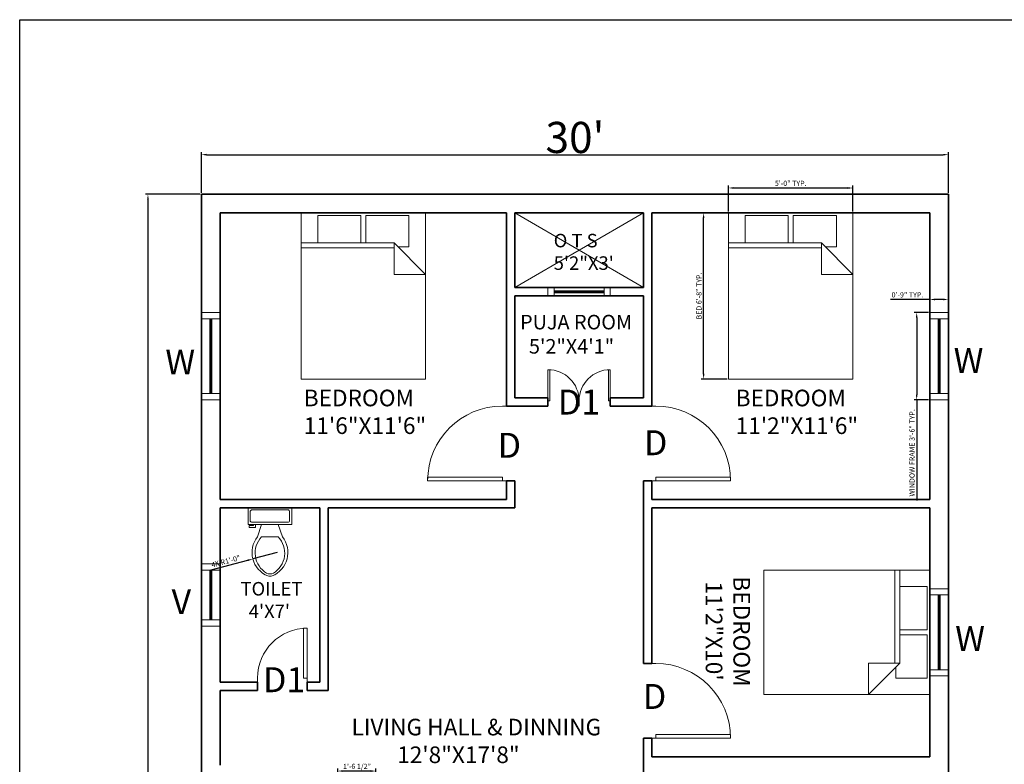
# Model space of a CAD drawing. Units: inches. Extents: x 2169 to 10664, y 1669 to 6352.
# Tile 4 of 17: x 2169 to 2644, y 2480 to 2838. Entities that reach past the tile are written whole.
import ezdxf

# ---------------------------------------------------------------- set-up
doc = ezdxf.new("R2010")
doc.units = ezdxf.units.IN
for name, color, linetype, lineweight in [('A-ANNO-DIMS', 3, 'Continuous', 18), ('A-ANNO-IDEN', 3, 'Continuous', 18), ('A-ANNO-SYMB', 6, 'Continuous', 13), ('A-ANNO-TTLB', 7, 'Continuous', 25), ('A-AREA-IDEN', 4, 'Continuous', 18), ('A-DOOR', 4, 'Continuous', 18), ('A-FLOR-FIXT', 9, 'Continuous', 18), ('A-FURN', 8, 'Continuous', 18), ('A-GLAZ', 30, 'Continuous', 18), ('A-WALL', 7, 'Continuous', 35)]:
    doc.layers.add(name, color=color, linetype=linetype, lineweight=lineweight)
doc.styles.get("Standard").update_dxf_attribs({"font": 'arial.ttf'})
doc.dimstyles.new('ISO-25', dxfattribs={"dimtxt": 2.5, "dimasz": 2.5, "dimexe": 1.25, "dimexo": 0.625, "dimtad": 1, "dimdec": 0, "dimlunit": 3, "dimtxsty": 'Standard', "dimcen": 2.5, "dimadec": 0, "dimazin": 0, "dimtfac": 1, "dimtdec": 0, "dimtmove": 0, "dimatfit": 3, "dimfxl": 1, "dimarcsym": 0})

# ---------------------------------------------------------------- blocks, each defined once
blk = doc.blocks.new('*U3')
for p, q in [((-24, 0), (-24, -6)), ((0, 0), (0, -6))]:
    blk.add_line(p, q)
blk.add_lwpolyline([(0, 0), (0, 24), (-1.75, 24), (-1.75, 0)], close=True)
blk.add_arc((0, 0), 24, 90, 180)
blk = doc.blocks.new('*U5')
for p, q in [((0, 0), (0, -6)), ((-36, 0), (-36, -6))]:
    blk.add_line(p, q)
blk.add_lwpolyline([(0, 0), (0, 36), (-1.75, 36), (-1.75, 0)], close=True)
blk.add_arc((0, 0), 36, 90, 180)
blk = doc.blocks.new('*U6')
for p, q in [((-36, 0), (-36, 6)), ((0, 0), (0, 6))]:
    blk.add_line(p, q)
blk.add_lwpolyline([(0, 0), (0, -36), (-1.75, -36), (-1.75, 0)], close=True)
blk.add_arc((0, 0), 36, 180, 270)
blk = doc.blocks.new('*U7')
for p, q in [((0, 0), (0, -6)), ((-36, 0), (-36, -6))]:
    blk.add_line(p, q)
blk.add_lwpolyline([(0, 0), (0, 36), (-1.75, 36), (-1.75, 0)], close=True)
blk.add_arc((0, 0), 36, 90, 180)
blk = doc.blocks.new('*U8')
for p, q in [((0, 0), (0, -5)), ((30, 0), (30, -5))]:
    blk.add_line(p, q)
blk.add_lwpolyline([(0, 0), (0, 30), (1.75, 30), (1.75, 0)], close=True)
blk.add_arc((0, 0), 30, 0, 90)
blk = doc.blocks.new('*U9')
for p, q in [((-30, 0), (-30, -5)), ((0, 0), (0, -5))]:
    blk.add_line(p, q)
blk.add_lwpolyline([(0, 0), (0, 30), (-1.75, 30), (-1.75, 0)], close=True)
blk.add_arc((0, 0), 30, 90, 180)
blk = doc.blocks.new('Bed - Queen')
for p, q in [((0, -80.00003), (0, 0)), ((0, 0), (59.99999, 0)), ((59.99999, 0), (59.99999, -80.00003)), ((7.99999, -1.2), (28.79998, -1.2)), ((7.99999, -14.4), (7.99999, -1.2)), ((28.79998, -1.2), (28.79998, -14.4)), ((31.19999, -1.2), (51.99999, -1.2)), ((31.19999, -14.4), (31.19999, -1.2)), ((51.99999, -1.2), (51.99999, -16.4)), ((0, -14.4), (44.8, -14.4)), ((44.8, -16.8), (0, -16.8)), ((59.99999, -29.6), (44.8, -14.4)), ((44.8, -14.4), (44.8, -29.6)), ((51.99999, -16.4), (46.79936, -16.4)), ((44.8, -29.6), (59.99999, -29.6)), ((59.99999, -80.00003), (0, -80.00003))]:
    blk.add_line(p, q)
blk = doc.blocks.new('Toilet - top')
for p, q in [((9.5, -6), (9.5, -2)), ((-10, -8.5), (-8, -8.5)), ((-10, -9.5), (-10, -8.5)), ((-8, -8.5), (-8, -8)), ((-7, -8), (-7, -9.5)), ((-4, -8), (-6, -14)), ((4, -8), (6, -14)), ((-7, -9.5), (-10, -9.5)), ((4, -14), (-4, -14))]:
    blk.add_line(p, q)
blk.add_lwpolyline([(10.5, -8), (10.5, 0), (-10.5, 0), (-10.5, -8)], close=True)
for points in [[(-9.5, -2), (-9.5, -6)], [(8.5, -1), (-8.5, -1)], [(-8.5, -7), (8.5, -7)]]:
    blk.add_lwpolyline(points)
for centre, radius, start, end in [((-8.62, -1.88), 0.884, 81.8699, 188.1301), ((8.62, -1.88), 0.884, 351.8699, 98.1301), ((-8.62, -6.12), 0.884, 171.8699, 278.1301), ((8.62, -6.12), 0.884, 261.8699, 8.1301), ((3.52, -21.58), 12.17, 141.4691, 247.9714), ((4.2, -21.82), 11.33, 136.3677, 238.9468), ((-3.52, -21.58), 12.17, 292.0284, 38.5307), ((-4.2, -21.82), 11.33, 301.053, 43.6321), ((0, -27.88), 4, 245.7318, 294.2682), ((0, -29), 4, 254.8605, 285.1395)]:
    blk.add_arc(centre, radius, start, end)
blk = doc.blocks.new('*D19')
at = {"layer": 'A-ANNO-DIMS', "color": 0, "lineweight": -2, "transparency": 16777216}
for p, q in [((2257.06, 2754.86), (2257.06, 2774.53)), ((2259.56, 2773.28), (2614.56, 2773.28)), ((2617.06, 2754.86), (2617.06, 2774.53))]:
    blk.add_line(p, q, dxfattribs=at)
at = {"layer": 'A-ANNO-DIMS', "color": 0, "transparency": 16777216}
for points in [[(2259.56, 2773.7), (2259.56, 2772.87), (2257.06, 2773.28)], [(2614.56, 2773.7), (2614.56, 2772.87), (2617.06, 2773.28)]]:
    blk.add_solid(points, dxfattribs=at)
at = {"layer": 'Defpoints', "color": 0, "transparency": 16777216}
for p in [(2617.06, 2773.28), (2257.06, 2754.23), (2617.06, 2754.23)]:
    blk.add_point(p, dxfattribs=at)
at = {"layer": 'A-ANNO-DIMS', "color": 0, "transparency": 16777216, "insert": (2437.06, 2781.57), "char_height": 2.5, "attachment_point": 5}
blk.add_mtext("{\\H6x;30'}", dxfattribs=at)
blk = doc.blocks.new('*D20')
at = {"layer": 'A-ANNO-DIMS', "color": 0, "lineweight": -2, "transparency": 16777216}
for p, q in [((2256.43, 2754.23), (2230.01, 2754.23)), ((2231.26, 2751.73), (2231.26, 2156.73)), ((2256.43, 2154.23), (2230.01, 2154.23))]:
    blk.add_line(p, q, dxfattribs=at)
at = {"layer": 'A-ANNO-DIMS', "color": 0, "transparency": 16777216}
for points in [[(2230.85, 2751.73), (2231.68, 2751.73), (2231.26, 2754.23)], [(2230.85, 2156.73), (2231.68, 2156.73), (2231.26, 2154.23)]]:
    blk.add_solid(points, dxfattribs=at)
at = {"layer": 'Defpoints', "color": 0, "transparency": 16777216}
for p in [(2257.06, 2754.23), (2231.26, 2154.23), (2257.06, 2154.23)]:
    blk.add_point(p, dxfattribs=at)
at = {"layer": 'A-ANNO-DIMS', "color": 0, "transparency": 16777216, "insert": (2222.98, 2454.23), "char_height": 2.5, "attachment_point": 5, "rotation": 90}
blk.add_mtext("{\\H6x;50'}", dxfattribs=at)
blk = doc.blocks.new('WIN-36-WALL-9')
for p, q in [((9, 42), (0, 42)), ((9, 39), (0, 39)), ((4, 39), (4, 3)), ((4.5, 39), (4.5, 3)), ((5, 39), (5, 3)), ((9, 3), (0, 3)), ((9, 0), (0, 0))]:
    blk.add_line(p, q)
blk = doc.blocks.new('WIN-24-WALL-9')
for p, q in [((9, 30), (0, 30)), ((9, 27), (0, 27)), ((4, 27), (4, 3)), ((4.5, 27), (4.5, 3)), ((5, 27), (5, 3)), ((9, 3), (0, 3)), ((9, 0), (0, 0))]:
    blk.add_line(p, q)
blk = doc.blocks.new('*D49')
at = {"layer": 'A-ANNO-DIMS', "color": 0, "lineweight": -2, "transparency": 16777216}
for p, q in [((2607.43, 2697.23), (2600.51, 2697.23)), ((2601.76, 2694.73), (2601.76, 2657.73)), ((2607.43, 2655.23), (2600.51, 2655.23)), ((2601.76, 2655.23), (2601.76, 2606.65))]:
    blk.add_line(p, q, dxfattribs=at)
at = {"layer": 'A-ANNO-DIMS', "color": 0, "transparency": 16777216}
for points in [[(2601.34, 2694.73), (2602.18, 2694.73), (2601.76, 2697.23)], [(2601.34, 2657.73), (2602.18, 2657.73), (2601.76, 2655.23)]]:
    blk.add_solid(points, dxfattribs=at)
at = {"layer": 'Defpoints', "color": 0, "transparency": 16777216}
for p in [(2608.06, 2697.23), (2601.76, 2655.23), (2608.06, 2655.23)]:
    blk.add_point(p, dxfattribs=at)
at = {"layer": 'A-ANNO-DIMS', "color": 0, "transparency": 16777216, "insert": (2599.84, 2629.69), "char_height": 2.5, "attachment_point": 5, "rotation": 90}
blk.add_mtext('WINDOW FRAME 3\'-6" TYP.', dxfattribs=at)
blk = doc.blocks.new('*D50')
at = {"layer": 'A-ANNO-DIMS', "color": 0, "lineweight": -2, "transparency": 16777216}
for p, q in [((2608.06, 2703.53), (2589.07, 2703.53)), ((2608.06, 2697.86), (2608.06, 2704.78)), ((2614.56, 2703.53), (2610.56, 2703.53)), ((2617.06, 2697.86), (2617.06, 2704.78))]:
    blk.add_line(p, q, dxfattribs=at)
at = {"layer": 'A-ANNO-DIMS', "color": 0, "transparency": 16777216}
for points in [[(2610.56, 2703.95), (2610.56, 2703.12), (2608.06, 2703.53)], [(2614.56, 2703.95), (2614.56, 2703.12), (2617.06, 2703.53)]]:
    blk.add_solid(points, dxfattribs=at)
at = {"layer": 'Defpoints', "color": 0, "transparency": 16777216}
for p in [(2608.06, 2703.53), (2608.06, 2697.23), (2617.06, 2697.23)]:
    blk.add_point(p, dxfattribs=at)
at = {"layer": 'A-ANNO-DIMS', "color": 0, "transparency": 16777216, "insert": (2597.31, 2705.44), "char_height": 2.5, "attachment_point": 5}
blk.add_mtext('0\'-9" TYP.', dxfattribs=at)
blk = doc.blocks.new('*D53')
at = {"layer": 'A-ANNO-DIMS', "color": 0, "lineweight": -2, "transparency": 16777216}
for p, q in [((2510.43, 2745.23), (2497.81, 2745.23)), ((2499.06, 2667.73), (2499.06, 2742.73)), ((2510.43, 2665.23), (2497.81, 2665.23))]:
    blk.add_line(p, q, dxfattribs=at)
at = {"layer": 'A-ANNO-DIMS', "color": 0, "transparency": 16777216}
for points in [[(2498.64, 2742.73), (2499.48, 2742.73), (2499.06, 2745.23)], [(2498.64, 2667.73), (2499.48, 2667.73), (2499.06, 2665.23)]]:
    blk.add_solid(points, dxfattribs=at)
at = {"layer": 'Defpoints', "color": 0, "transparency": 16777216}
for p in [(2499.06, 2745.23), (2511.06, 2745.23), (2511.06, 2665.23)]:
    blk.add_point(p, dxfattribs=at)
at = {"layer": 'A-ANNO-DIMS', "color": 0, "transparency": 16777216, "insert": (2497.16, 2705.23), "char_height": 2.5, "attachment_point": 5, "rotation": 90}
blk.add_mtext('BED 6\'-8" TYP.', dxfattribs=at)
blk = doc.blocks.new('*D54')
at = {"layer": 'A-ANNO-DIMS', "color": 0, "lineweight": -2, "transparency": 16777216}
for p, q in [((2511.06, 2745.86), (2511.06, 2758.48)), ((2513.56, 2757.23), (2568.56, 2757.23)), ((2571.06, 2745.86), (2571.06, 2758.48))]:
    blk.add_line(p, q, dxfattribs=at)
at = {"layer": 'A-ANNO-DIMS', "color": 0, "transparency": 16777216}
for points in [[(2513.56, 2757.65), (2513.56, 2756.82), (2511.06, 2757.23)], [(2568.56, 2757.65), (2568.56, 2756.82), (2571.06, 2757.23)]]:
    blk.add_solid(points, dxfattribs=at)
at = {"layer": 'Defpoints', "color": 0, "transparency": 16777216}
for p in [(2571.06, 2757.23), (2511.06, 2745.23), (2571.06, 2745.23)]:
    blk.add_point(p, dxfattribs=at)
at = {"layer": 'A-ANNO-DIMS', "color": 0, "transparency": 16777216, "insert": (2541.06, 2759.14), "char_height": 2.5, "attachment_point": 5}
blk.add_mtext('5\'-0" TYP.', dxfattribs=at)
blk = doc.blocks.new('*D62')
at = {"layer": 'A-ANNO-DIMS', "color": 0, "lineweight": -2, "transparency": 16777216}
for p, q in [((2322.83, 2470.75), (2322.83, 2477.68)), ((2341.17, 2470.75), (2341.17, 2477.68)), ((2338.67, 2476.43), (2325.33, 2476.43))]:
    blk.add_line(p, q, dxfattribs=at)
at = {"layer": 'A-ANNO-DIMS', "color": 0, "transparency": 16777216}
for points in [[(2325.33, 2476.85), (2325.33, 2476.01), (2322.83, 2476.43)], [(2338.67, 2476.85), (2338.67, 2476.01), (2341.17, 2476.43)]]:
    blk.add_solid(points, dxfattribs=at)
at = {"layer": 'Defpoints', "color": 0, "transparency": 16777216}
for p in [(2322.83, 2476.43), (2322.83, 2470.13), (2341.17, 2470.13)]:
    blk.add_point(p, dxfattribs=at)
at = {"layer": 'A-ANNO-DIMS', "color": 0, "transparency": 16777216, "insert": (2332, 2478.35), "char_height": 2.5, "attachment_point": 5}
blk.add_mtext('1\'-6 1/2"', dxfattribs=at)
blk = doc.blocks.new('*D134')
at = {"layer": 'A-ANNO-DIMS', "color": 0, "lineweight": -2, "transparency": 16777216}
for p, q in [((2293.58, 2581.65), (2281.81, 2578.56)), ((2261.73, 2573.29), (2279.39, 2577.93))]:
    blk.add_line(p, q, dxfattribs=at)
at = {"layer": 'A-ANNO-DIMS', "color": 0, "transparency": 16777216}
blk.add_solid([(2279.29, 2578.33), (2279.5, 2577.52), (2281.81, 2578.56)], dxfattribs=at)
at = {"layer": 'Defpoints', "color": 0, "transparency": 16777216}
for p in [(2293.58, 2581.65), (2281.81, 2578.56)]:
    blk.add_point(p, dxfattribs=at)
at = {"layer": 'A-ANNO-DIMS', "color": 0, "transparency": 16777216, "insert": (2268.87, 2577.13), "char_height": 2.5, "attachment_point": 5, "rotation": 14.7211}
blk.add_mtext('4X R1\'-0"', dxfattribs=at)

msp = doc.modelspace()

# ---------------------------------------------------------------- linework, layer by layer
at = {"layer": 'A-ANNO-SYMB'}
for p, q in [((2408.06, 2709.23), (2470.06, 2745.23)), ((2408.06, 2745.23), (2470.06, 2709.23))]:
    msp.add_line(p, q, dxfattribs=at)
at = {"layer": 'A-ANNO-TTLB'}
msp.add_lwpolyline([(2169.45, 2838.28), (3251.13, 2838.28), (3251.13, 1669.34), (2169.45, 1669.34)], close=True, dxfattribs=at)
at = {"layer": 'A-GLAZ'}
for p, q in [((2424.06, 2705.23), (2424.06, 2709.23)), ((2427.06, 2705.23), (2427.06, 2709.23)), ((2427.06, 2707.73), (2451.06, 2707.73)), ((2427.06, 2707.23), (2451.06, 2707.23)), ((2427.06, 2706.73), (2451.06, 2706.73)), ((2451.06, 2705.23), (2451.06, 2709.23)), ((2454.06, 2705.23), (2454.06, 2709.23))]:
    msp.add_line(p, q, dxfattribs=at)
at = {"layer": 'A-WALL'}
for p, q in [((2257.06, 2754.23), (2617.06, 2754.23)), ((2257.06, 2154.23), (2257.06, 2754.23)), ((2617.06, 2754.23), (2617.06, 2154.23)), ((2266.06, 2745.23), (2404.06, 2745.23)), ((2266.06, 2607.23), (2266.06, 2745.23)), ((2404.06, 2652.23), (2404.06, 2745.23)), ((2408.06, 2745.23), (2470.06, 2745.23)), ((2408.06, 2709.23), (2408.06, 2745.23)), ((2470.06, 2709.23), (2470.06, 2745.23)), ((2474.06, 2745.23), (2608.06, 2745.23)), ((2474.06, 2652.23), (2474.06, 2745.23)), ((2608.06, 2745.23), (2608.06, 2607.23)), ((2408.06, 2709.23), (2470.06, 2709.23)), ((2408.06, 2656.23), (2408.06, 2705.23)), ((2408.06, 2705.23), (2470.06, 2705.23)), ((2470.06, 2656.23), (2470.06, 2705.23)), ((2408.06, 2656.23), (2408.06, 2699.23)), ((2470.06, 2656.23), (2470.06, 2699.23)), ((2408.06, 2656.23), (2424.06, 2656.23)), ((2424.06, 2656.23), (2424.06, 2652.23)), ((2454.06, 2656.23), (2470.06, 2656.23)), ((2454.06, 2656.23), (2454.06, 2652.23)), ((2404.06, 2652.23), (2424.06, 2652.23)), ((2454.06, 2652.23), (2470.06, 2652.23)), ((2470.06, 2652.23), (2474.06, 2652.23)), ((2404.06, 2607.23), (2404.06, 2616.23)), ((2404.06, 2616.23), (2408.06, 2616.23)), ((2408.06, 2603.23), (2408.06, 2616.23)), ((2470.06, 2528.23), (2470.06, 2616.23)), ((2470.06, 2616.23), (2474.06, 2616.23)), ((2474.06, 2607.23), (2474.06, 2616.23)), ((2266.06, 2607.23), (2281.06, 2607.23)), ((2281.06, 2607.23), (2404.06, 2607.23)), ((2474.06, 2607.23), (2608.06, 2607.23)), ((2266.06, 2519.23), (2266.06, 2603.23)), ((2266.06, 2603.23), (2314.06, 2603.23)), ((2314.06, 2519.23), (2314.06, 2603.23)), ((2318.06, 2515.23), (2318.06, 2603.23)), ((2318.06, 2603.23), (2408.06, 2603.23)), ((2474.06, 2603.23), (2608.06, 2603.23)), ((2474.06, 2528.23), (2474.06, 2603.23)), ((2608.06, 2603.23), (2608.06, 2483.23)), ((2470.06, 2528.23), (2474.06, 2528.23)), ((2266.06, 2519.23), (2284.06, 2519.23)), ((2266.06, 2515.23), (2284.06, 2515.23)), ((2266.06, 2479.23), (2266.06, 2515.23)), ((2284.06, 2515.23), (2284.06, 2519.23)), ((2308.06, 2515.23), (2308.06, 2519.23)), ((2308.06, 2519.23), (2314.06, 2519.23)), ((2308.06, 2515.23), (2318.06, 2515.23)), ((2470.06, 2470.23), (2470.06, 2492.23)), ((2470.06, 2492.23), (2474.06, 2492.23)), ((2474.06, 2483.23), (2474.06, 2492.23)), ((2474.06, 2483.23), (2608.06, 2483.23))]:
    msp.add_line(p, q, dxfattribs=at)

# ---------------------------------------------------------------- block references
at = {"layer": 'A-DOOR', "xscale": 0.5, "yscale": 0.5, "zscale": 0.5}
for name, p in [('*U8', (2424.06, 2654.73)), ('*U9', (2454.06, 2654.73))]:
    msp.add_blockref(name, p, dxfattribs=at)
at = {"layer": 'A-DOOR', "rotation": 270}
for name, p in [('*U6', (2402.06, 2616.23)), ('*U7', (2476.06, 2616.23)), ('*U5', (2476.06, 2492.23))]:
    msp.add_blockref(name, p, dxfattribs=at)
at = {"layer": 'A-DOOR'}
msp.add_blockref('*U3', (2308.06, 2521.23), dxfattribs=at)
at = {"layer": 'A-FLOR-FIXT'}
msp.add_blockref('Toilet - top', (2290.06, 2603.23), dxfattribs=at)
at = {"layer": 'A-FURN'}
for p in [(2305.06, 2745.23), (2511.06, 2745.23)]:
    msp.add_blockref('Bed - Queen', p, dxfattribs=at)
at = {"layer": 'A-FURN', "rotation": 270}
msp.add_blockref('Bed - Queen', (2608.06, 2573.23), dxfattribs=at)
at = {"layer": 'A-GLAZ'}
for name, p in [('WIN-36-WALL-9', (2257.06, 2655.23)), ('WIN-24-WALL-9', (2257.06, 2546.23))]:
    msp.add_blockref(name, p, dxfattribs=at)
at = {"layer": 'A-GLAZ', "rotation": 180}
for p in [(2617.06, 2697.23), (2617.06, 2564.23)]:
    msp.add_blockref('WIN-36-WALL-9', p, dxfattribs=at)

# ---------------------------------------------------------------- texts
at = {"layer": 'A-ANNO-IDEN', "char_height": 12, "attachment_point": 1}
for s, insert in [('W', (2239.64, 2679.44)), ('W', (2619.56, 2680.2)), ('D1', (2428.8, 2660.12)), ('D', (2399.8, 2639.3)), ('D', (2470.33, 2640.53)), ('V', (2242.65, 2563.99)), ('W', (2620.3, 2546.28)), ('D1', (2286.73, 2526.41)), ('D', (2469.81, 2518.34))]:
    msp.add_mtext_dynamic_manual_height_columns(s, width=497.3673, gutter_width=12.5, heights=[0], dxfattribs=dict(at, insert=insert))
at = {"layer": 'A-AREA-IDEN', "attachment_point": 1}
for s, width, insert, char_height in [('O T S\\P5\'2"X3\'', 234.9563, (2426.82, 2735.15), 6.5), ('PUJA ROOM\\P  5\'2"X4\'1"', 218.0912, (2410.61, 2696.14), 7), ('BEDROOM\\P11\'6"X11\'6"', 532.8762, (2306.37, 2660.1), 8), ('BEDROOM\\P11\'2"X11\'6"', 532.8762, (2514.53, 2660.09), 8), ("TOILET\\P  4'X7'", 196.7478, (2275.88, 2567.46), 6.5), ('LIVING HALL & DINNING\\P         12\'8"X17\'8"', 652.2569, (2329.38, 2501.6), 8)]:
    msp.add_mtext_dynamic_manual_height_columns(s, width=width, gutter_width=12.5, heights=[0], dxfattribs=dict(at, insert=insert, char_height=char_height))
at = {"layer": 'A-AREA-IDEN', "insert": (2521.42, 2570.2), "char_height": 8, "attachment_point": 1, "rotation": 270}
msp.add_mtext_dynamic_manual_height_columns('BEDROOM\\P 11\'2"X10\'', width=532.8762, gutter_width=12.5, heights=[0], dxfattribs=at)

# ---------------------------------------------------------------- dimensions: what is measured, and where the dimension line sits
at = {"layer": 'A-ANNO-DIMS'}
for base, p1, p2, text, override, picture, middle in [((2617.06, 2773.28), (2257.06, 2754.23), (2617.06, 2754.23), '{\\H6x;<>}', {"dimclrd": 0, "dimclre": 0, "dimclrt": 0}, '*D19', (2437.06, 2781.57)), ((2571.06, 2757.23), (2511.06, 2745.23), (2571.06, 2745.23), '<> TYP.', {"dimdec": 1, "dimlfac": 1, "dimrnd": 0, "dimzin": 1, "dimdsep": 46, "dimlunit": 4, "dimfrac": 2}, '*D54', (2541.06, 2759.14))]:
    dim = msp.add_linear_dim(base=base, p1=p1, p2=p2, text=text, dimstyle='ISO-25', override=override, dxfattribs=at)
    dim.commit()
    dim.dimension.update_dxf_attribs({"geometry": picture, "text_midpoint": middle})
for base, p1, p2, angle, text, override, picture, middle in [((2231.26, 2154.23), (2257.06, 2754.23), (2257.06, 2154.23), 90, '{\\H6x;<>}', {"dimclrd": 0, "dimclre": 0, "dimclrt": 0}, '*D20', (2222.98, 2454.23)), ((2499.06, 2745.23), (2511.06, 2665.23), (2511.06, 2745.23), 90, 'BED <> TYP.', {"dimdec": 1, "dimlfac": 1, "dimrnd": 0, "dimzin": 1, "dimdsep": 46, "dimlunit": 4, "dimfrac": 2}, '*D53', (2497.16, 2705.23)), ((2608.06, 2703.53), (2617.06, 2697.23), (2608.06, 2697.23), 180, '<> TYP.', {"dimdec": 1, "dimlfac": 1, "dimrnd": 0, "dimzin": 1, "dimdsep": 46, "dimlunit": 4, "dimfrac": 2}, '*D50', (2597.31, 2705.44)), ((2601.76, 2655.23), (2608.06, 2697.23), (2608.06, 2655.23), 270, 'WINDOW FRAME <> TYP.', {"dimdec": 1, "dimlfac": 1, "dimrnd": 0, "dimzin": 1, "dimdsep": 46, "dimlunit": 4, "dimfrac": 2}, '*D49', (2599.84, 2629.69))]:
    dim = msp.add_linear_dim(base=base, p1=p1, p2=p2, angle=angle, text=text, dimstyle='ISO-25', override=override, dxfattribs=at)
    dim.commit()
    dim.dimension.update_dxf_attribs({"geometry": picture, "text_midpoint": middle})
dim = msp.add_radius_dim(center=(2293.58, 2581.65), mpoint=(2281.81, 2578.56), text='4X <>', dimstyle='ISO-25', override={"dimdec": 1, "dimlfac": 1, "dimrnd": 0, "dimzin": 1, "dimdsep": 46, "dimlunit": 4, "dimfrac": 2}, dxfattribs=at)
dim.commit()
dim.dimension.update_dxf_attribs({"geometry": '*D134', "text_midpoint": (2268.87, 2577.13)})
dim = msp.add_linear_dim(base=(2322.83, 2476.43), p1=(2341.17, 2470.13), p2=(2322.83, 2470.13), angle=180, dimstyle='ISO-25', override={"dimdec": 1, "dimlfac": 1, "dimrnd": 0, "dimzin": 1, "dimdsep": 46, "dimlunit": 4, "dimfrac": 2}, dxfattribs=at)
dim.commit()
dim.dimension.update_dxf_attribs({"geometry": '*D62', "text_midpoint": (2332, 2478.35)})

doc.saveas('drawing.dxf')
